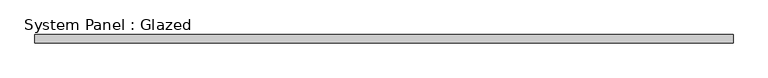
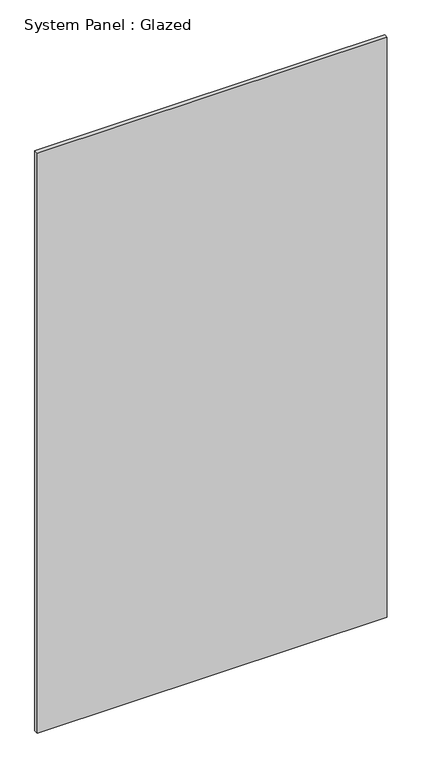
"""IFC4 building model written with IfcOpenShell, lengths in millimetres: plate geometry, System Panel : Glazed."""

from ifc_helpers import new_model, si_unit, origin, origin_with_axes, place, context, project, spatial, polyline, outline, extrude, source, transform, mapped, element, save


def system_panel_glazed_da3fd9d5(model_context):
    return source(origin(), model_context, "Body", "SweptSolid", [
        extrude(outline(polyline([(1095.375, 19.05), (-1095.375, 19.05), (-1095.375, 44.45), (1095.375, 44.45), (1095.375, 19.05)])), origin_with_axes(), (0.0, 0.0, 1.0), 3835.4),
    ])


if __name__ == "__main__":
    model = new_model("IFC4")
    model_context = context("Model", 3, world=origin())
    ifc_project = project(units=[si_unit("LENGTHUNIT", "METRE", prefix="MILLI")], contexts=[model_context])
    site = spatial("IfcSite", under=ifc_project)
    building = spatial("IfcBuilding", under=site)
    placement = place(None, origin())
    system_panel_glazed_shape = system_panel_glazed_da3fd9d5(model_context)
    element("IfcPlate", 1, ObjectType="System Panel : Glazed", at=placement, inside=building, context=model_context, shape_type="MappedRepresentation", body=[
        mapped(system_panel_glazed_shape, transform((0.0, 0.0, 0.0), x_axis=(1.0, 0.0, 0.0), y_axis=(0.0, 1.0, 0.0), z_axis=(0.0, 0.0, 1.0))),
    ])
    save(model, "model.ifc")

# Revit data of these elements
# Type "System Panel : Glazed"
#   Construction Type Id = "GSP4R"
#   Analytic Construction = "1/8 in Pilkington single glazing"
#   Visual Light Transmittance = 0.9
#   Solar Heat Gain Coefficient = 0.86
#   Heat Transfer Coefficient (U) = 1.18115 BTU/(h·ft²·°F)
# Element 1 (IfcPlate, "System Panel : Glazed")
#   Materials on its faces: "Glass"
# Materials
#   "Glass": class "Glass", colour RGB 0 128 192, transparency 0.75, Description = "Soda Lime Glass", Cost = 0
